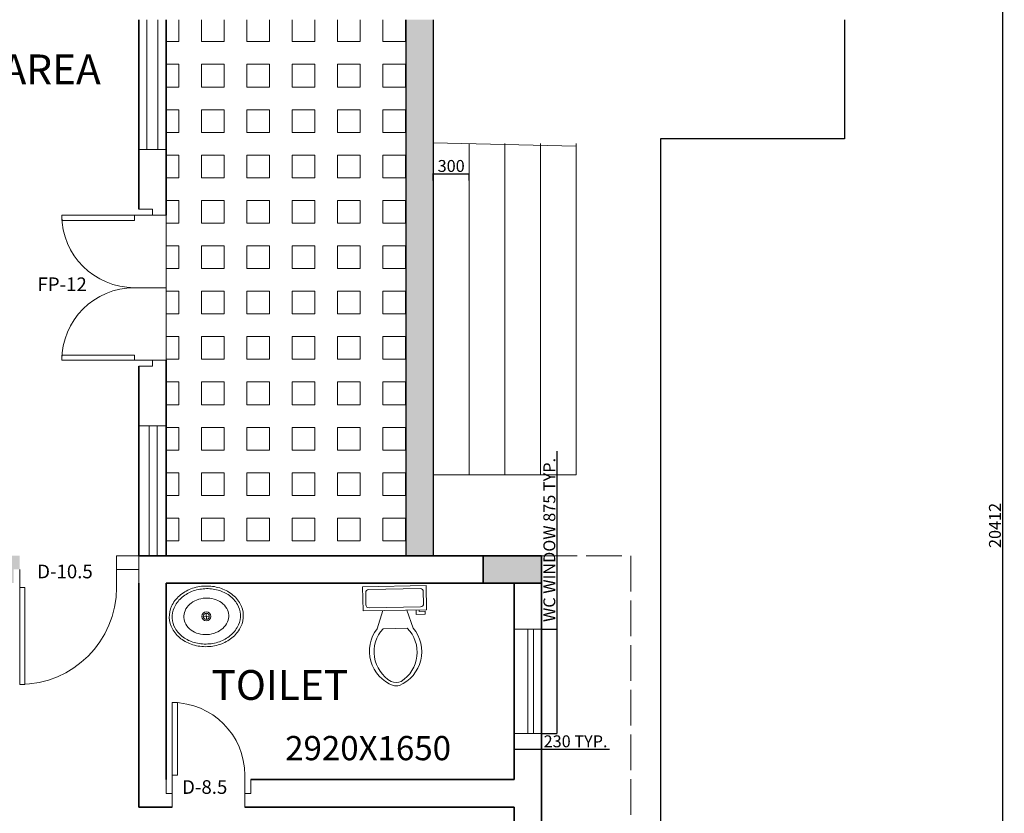
# Model space of a CAD drawing. Units: millimetres. Extents: x -17016 to 4866, y -18325 to 4338.
# Tile 4 of 5: x -3399 to 4866, y -9462 to -2799. Entities that reach past the tile are written whole.
import ezdxf

# ---------------------------------------------------------------- set-up
doc = ezdxf.new("R2010")
doc.units = ezdxf.units.MM
doc.header["$LTSCALE"] = 5
doc.linetypes.add('ACAD_ISO02W100', pattern=[15, 12, -3])
for name, color, linetype, lineweight in [('A-ANNO-DIMS', 2, 'Continuous', 18), ('A-ANNO-IDEN', 3, 'Continuous', 18), ('A-AREA-IDEN', 7, 'Continuous', 25), ('A-COLS', 7, 'Continuous', 35), ('A-COLS-PATT', 252, 'Continuous', 13), ('A-DOOR', 3, 'Continuous', 18), ('A-FLOR-FIXT', 9, 'Continuous', 18), ('A-FLOR-OTLN', 8, 'Continuous', 25), ('A-FLOR-PATT', 252, 'Continuous', 13), ('A-FLOR-STRS', 7, 'Continuous', 18), ('A-GLAZ', 4, 'Continuous', 18), ('A-ROOF-OVHD', 8, 'ACAD_ISO02W100', 13), ('A-WALL', 7, 'Continuous', 35)]:
    doc.layers.add(name, color=color, linetype=linetype, lineweight=lineweight)
doc.styles.get("Standard").update_dxf_attribs({"font": 'arial.ttf'})
doc.dimstyles.new('Copy of ISO-25', dxfattribs={"dimtxt": 100, "dimasz": 2.5, "dimexe": 1.25, "dimexo": 0.625, "dimtad": 1, "dimdec": 0, "dimtxsty": 'Standard', "dimcen": 2.5, "dimadec": 0, "dimazin": 0, "dimtfac": 1, "dimtdec": 0, "dimtmove": 0, "dimatfit": 3, "dimfxl": 1, "dimarcsym": 0})

# ---------------------------------------------------------------- blocks, each defined once
blk = doc.blocks.new('*U3')
for p, q in [((0, 0), (0, -6)), ((24, 0), (24, -6))]:
    blk.add_line(p, q)
blk.add_lwpolyline([(0, 0), (0, 24), (1.75, 24), (1.75, 0)], close=True)
blk.add_arc((0, 0), 24, 0, 90)
blk = doc.blocks.new('Sink - Oval top')
for p, q in [((-1, 0), (1, 0)), ((0, 1), (0, -1))]:
    blk.add_line(p, q)
for points in [[(-12.23, 0.39, 0.117634), (-11.46, -3.36, 0.104469), (-8.88, -6.8, 0.090016), (-5.08, -9.07, 0.08192), (-0.32, -10.02, 0.08192), (4.49, -9.38, 0.090016), (8.42, -7.36, 0.104469), (11.22, -4.09, 0.117634), (12.23, -0.39, 0.117634), (11.46, 3.36, 0.104469), (8.88, 6.8, 0.090016), (5.08, 9.07, 0.08192), (0.32, 10.02, 0.08192), (-4.49, 9.38, 0.090016), (-8.42, 7.36, 0.104469), (-11.22, 4.09, 0.117634)], [(-11.29, 0.16, 0.118622), (-10.52, -3.25, 0.104678), (-8.07, -6.36, 0.089562), (-4.54, -8.37, 0.081185), (-0.13, -9.15, 0.081185), (4.3, -8.49, 0.089562), (7.89, -6.58, 0.104678), (10.42, -3.55, 0.118622), (11.29, -0.16, 0.118622), (10.52, 3.25, 0.104678), (8.07, 6.36, 0.089562), (4.54, 8.37, 0.081185), (0.13, 9.15, 0.081185), (-4.3, 8.49, 0.089562), (-7.89, 6.58, 0.104678), (-10.42, 3.55, 0.118622)], [(-7.42, 0.08, 0.118283), (-6.91, -2.17, 0.104607), (-5.29, -4.21, 0.089718), (-2.97, -5.53, 0.081436), (-0.07, -6.04, 0.081436), (2.84, -5.59, 0.089718), (5.2, -4.33, 0.104607), (6.86, -2.32, 0.118283), (7.42, -0.08, 0.118283), (6.91, 2.17, 0.104607), (5.29, 4.21, 0.089718), (2.97, 5.53, 0.081436), (0.07, 6.04, 0.081436), (-2.84, 5.59, 0.089718), (-5.2, 4.33, 0.104607), (-6.86, 2.32, 0.118283)]]:
    blk.add_lwpolyline(points, format="xyb", close=True)
for radius in [1.5, 1]:
    blk.add_circle((0, 0), radius)
blk = doc.blocks.new('*U13')
for p, q in [((9.5, -6), (9.5, -2)), ((-10, -8.5), (-8, -8.5)), ((-10, -9.5), (-10, -8.5)), ((-7, -9.5), (-10, -9.5)), ((-8, -8.5), (-8, -8)), ((-7, -8), (-7, -9.5)), ((-4, -8), (-6, -14)), ((4, -8), (6, -14)), ((4, -14), (-4, -14))]:
    blk.add_line(p, q)
blk.add_lwpolyline([(10.5, -8), (10.5, 0), (-10.5, 0), (-10.5, -8)], close=True)
for points in [[(-9.5, -2), (-9.5, -6)], [(8.5, -1), (-8.5, -1)], [(-8.5, -7), (8.5, -7)]]:
    blk.add_lwpolyline(points)
for centre, radius, start, end in [((-8.62, -1.88), 0.884, 81.8699, 188.1301), ((8.62, -1.88), 0.884, 351.8699, 98.1301), ((-8.62, -6.12), 0.884, 171.8699, 278.1301), ((8.62, -6.12), 0.884, 261.8699, 8.1301), ((3.52, -21.58), 12.17, 141.4691, 247.9714), ((4.2, -21.82), 11.33, 136.3677, 238.9468), ((-3.52, -21.58), 12.17, 292.0284, 38.5307), ((-4.2, -21.82), 11.33, 301.053, 43.6321), ((0, -27.88), 4, 245.7318, 294.2682), ((0, -29), 4, 254.8605, 285.1395)]:
    blk.add_arc(centre, radius, start, end)
blk = doc.blocks.new('*U2')
for p, q in [((0, 0), (0, -6)), ((32, 0), (32, -6))]:
    blk.add_line(p, q)
blk.add_lwpolyline([(0, 0), (0, 32), (1.75, 32), (1.75, 0)], close=True)
blk.add_arc((0, 0), 32, 0, 90)
blk = doc.blocks.new('*D16')
at = {"layer": 'A-ANNO-DIMS', "color": 0, "lineweight": -2, "ltscale": 5, "transparency": 16777216}
for p, q in [((72.8, -4147.8), (72.8, -4090.5)), ((75.3, -4091.8), (370.2, -4091.8)), ((372.7, -4147.8), (372.7, -4090.5))]:
    blk.add_line(p, q, dxfattribs=at)
at = {"layer": 'A-ANNO-DIMS', "color": 0, "ltscale": 5, "transparency": 16777216}
for points in [[(75.3, -4091.4), (75.3, -4092.2), (72.8, -4091.8)], [(370.2, -4091.4), (370.2, -4092.2), (372.7, -4091.8)]]:
    blk.add_solid(points, dxfattribs=at)
at = {"layer": 'Defpoints', "color": 0, "ltscale": 5, "transparency": 16777216}
for p in [(372.7, -4091.8), (72.8, -4148.4), (372.7, -4148.4)]:
    blk.add_point(p, dxfattribs=at)
at = {"layer": 'A-ANNO-DIMS', "color": 0, "ltscale": 5, "transparency": 16777216, "insert": (222.8, -4040.1), "char_height": 100, "attachment_point": 5}
blk.add_mtext('300', dxfattribs=at)
blk = doc.blocks.new('WIN-TOILET-875')
for p, q in [((0, 874.8), (230, 874.8)), ((115, 874.8), (115, 0)), ((164.3, 874.8), (164.3, 0)), ((0, 0), (230, 0))]:
    blk.add_line(p, q)
blk = doc.blocks.new('*D34')
at = {"layer": 'A-ANNO-DIMS', "color": 0, "lineweight": -2, "ltscale": 5, "transparency": 16777216}
for p, q in [((1112, -7915.9), (1112, -6420.3)), ((981.4, -7915.9), (1113.3, -7915.9)), ((1112, -8788.2), (1112, -7918.4)), ((981.4, -8790.7), (1113.3, -8790.7))]:
    blk.add_line(p, q, dxfattribs=at)
at = {"layer": 'A-ANNO-DIMS', "color": 0, "ltscale": 5, "transparency": 16777216}
for points in [[(1111.6, -7918.4), (1112.5, -7918.4), (1112, -7915.9)], [(1111.6, -8788.2), (1112.5, -8788.2), (1112, -8790.7)]]:
    blk.add_solid(points, dxfattribs=at)
at = {"layer": 'Defpoints', "color": 0, "ltscale": 5, "transparency": 16777216}
for p in [(980.8, -7915.9), (1112, -7915.9), (980.8, -8790.7)]:
    blk.add_point(p, dxfattribs=at)
at = {"layer": 'A-ANNO-DIMS', "color": 0, "ltscale": 5, "transparency": 16777216, "insert": (1059.7, -7166.8), "char_height": 100, "attachment_point": 5, "rotation": 90}
blk.add_mtext('WC WINDOW 875 TYP.', dxfattribs=at)
blk = doc.blocks.new('*D35')
at = {"layer": 'A-ANNO-DIMS', "color": 0, "lineweight": -2, "ltscale": 5, "transparency": 16777216}
for p, q in [((750.8, -8791.3), (750.8, -8923.1)), ((980.8, -8791.3), (980.8, -8923.1)), ((753.3, -8921.9), (978.3, -8921.9)), ((980.8, -8921.9), (1550.7, -8921.9))]:
    blk.add_line(p, q, dxfattribs=at)
at = {"layer": 'A-ANNO-DIMS', "color": 0, "ltscale": 5, "transparency": 16777216}
for points in [[(753.3, -8921.5), (753.3, -8922.3), (750.8, -8921.9)], [(978.3, -8921.5), (978.3, -8922.3), (980.8, -8921.9)]]:
    blk.add_solid(points, dxfattribs=at)
at = {"layer": 'Defpoints', "color": 0, "ltscale": 5, "transparency": 16777216}
for p in [(750.8, -8790.7), (980.8, -8790.7), (980.8, -8921.9)]:
    blk.add_point(p, dxfattribs=at)
at = {"layer": 'A-ANNO-DIMS', "color": 0, "ltscale": 5, "transparency": 16777216, "insert": (1267, -8870.2), "char_height": 100, "attachment_point": 5}
blk.add_mtext('230 TYP.', dxfattribs=at)
blk = doc.blocks.new('*D47')
at = {"layer": 'A-ANNO-DIMS', "color": 0, "lineweight": -2, "ltscale": 5, "transparency": 16777216}
for p, q in [((3524.2, 3160.9), (4853.2, 3160.9)), ((4851.9, 3158.4), (4851.9, -17248.3)), ((-3159.9, -17250.8), (4853.2, -17250.8))]:
    blk.add_line(p, q, dxfattribs=at)
at = {"layer": 'A-ANNO-DIMS', "color": 0, "ltscale": 5, "transparency": 16777216}
for points in [[(4851.5, 3158.4), (4852.3, 3158.4), (4851.9, 3160.9)], [(4851.5, -17248.3), (4852.3, -17248.3), (4851.9, -17250.8)]]:
    blk.add_solid(points, dxfattribs=at)
at = {"layer": 'Defpoints', "color": 0, "ltscale": 5, "transparency": 16777216}
for p in [(3523.6, 3160.9), (-3160.5, -17250.8), (4851.9, -17250.8)]:
    blk.add_point(p, dxfattribs=at)
at = {"layer": 'A-ANNO-DIMS', "color": 0, "ltscale": 5, "transparency": 16777216, "insert": (4800.2, -7045), "char_height": 100, "attachment_point": 5, "rotation": 90}
blk.add_mtext('20412', dxfattribs=at)

msp = doc.modelspace()

# ---------------------------------------------------------------- hatches: boundary and pattern name
at = {"layer": 'A-COLS-PATT', "ltscale": 5}
h = msp.add_hatch(color=256, dxfattribs=at)
h.dxf.hatch_style = 1
h.paths.add_polyline_path([(980.82, -7299.11), (490.82, -7299.11), (490.82, -7529.11), (980.82, -7529.11)])
h.paths.add_polyline_path([(-3449.18, -7414.11), (-3399.18, -7414.11), (-3399.18, -7299.11), (-3939.18, -7299.11), (-3939.18, -7529.11), (-3449.18, -7529.11)])
h.paths.add_polyline_path([(-8219.18, -7299.11), (-8709.18, -7299.11), (-8709.18, -7529.11), (-8219.18, -7529.11)])
h.paths.add_polyline_path([(-12649.22, -7299.11), (-13139.18, -7299.11), (-13139.18, -7529.11), (-12649.22, -7529.11)])
at = {"layer": 'A-FLOR-PATT'}
h = msp.add_hatch(dxfattribs=at)
h.set_pattern_fill('ANGLE', color=256, scale=25)
h.set_pattern_definition([(0, (-20162.07, -7174.37), (0, 174.625), [127, -47.625]), (90, (-20162.07, -7174.37), (-174.625, 1e-14), [127, -47.625])])
h.paths.add_polyline_path([(72.82, -2799.11), (-157.18, -2799.11), (-157.18, -7299.11), (72.82, -7299.11)])
h.paths.add_polyline_path([(-12231.38, -2799.11), (-12461.38, -2799.11), (-12461.38, -7299.11), (-12231.38, -7299.11)])
h = msp.add_hatch(dxfattribs=at)
h.set_pattern_fill('SQUARE', color=256, scale=60)
h.set_pattern_definition([(0, (-20162.07, -7174.37), (0, 190.5), [190.5, -190.5]), (90, (-20162.07, -7174.37), (-190.5, 1e-14), [190.5, -190.5])])
h.paths.add_polyline_path([(-157.18, -2799.11), (-436.38, -2799.11), (-2169.18, -2799.11), (-2169.18, -4439.51), (-2169.18, -5658.71), (-2169.18, -7299.11), (-157.18, -7299.11)])
h.paths.add_polyline_path([(-9989.18, -4439.51), (-9989.18, -2799.11), (-12231.38, -2799.11), (-12231.38, -7299.11), (-9989.18, -7299.11), (-9989.18, -5658.71)])

# ---------------------------------------------------------------- linework, layer by layer
at = {"layer": 'A-COLS', "ltscale": 5}
msp.add_line((490.82, -7534.51), (490.82, -7299.11), dxfattribs=at)
at = {"layer": 'A-DOOR'}
for p, q in [((-2284.18, -4389.51), (-2399.18, -4389.51)), ((-2284.18, -4439.51), (-2284.18, -4389.51)), ((-2284.18, -4439.51), (-2169.18, -4439.51)), ((-2169.18, -4439.51), (-2169.18, -5658.71)), ((-2399.18, -5049.11), (-2169.18, -5049.11)), ((-2284.18, -5658.71), (-2284.18, -5708.71)), ((-2284.18, -5658.71), (-2169.18, -5658.71)), ((-2284.18, -5708.71), (-2399.18, -5708.71)), ((-2586.38, -7414.11), (-2586.38, -7299.11)), ((-2399.18, -7299.11), (-2586.38, -7299.11)), ((-2399.18, -7299.11), (-2399.18, -7529.11)), ((-2586.38, -7414.11), (-2399.18, -7414.11)), ((-2169.18, -9179.11), (-2169.18, -9294.11)), ((-1459.58, -9294.11), (-1459.58, -9179.11)), ((-2169.18, -9294.11), (-2119.18, -9294.11)), ((-2119.18, -9294.11), (-2119.18, -9409.11)), ((-1509.58, -9294.11), (-1459.58, -9294.11)), ((-1509.58, -9294.11), (-1509.58, -9409.11))]:
    msp.add_line(p, q, dxfattribs=at)
at = {"layer": 'A-FLOR-OTLN'}
for p, q in [((-157.18, -2799.11), (-157.18, -7299.11)), ((72.82, -2799.11), (72.82, -7299.11))]:
    msp.add_line(p, q, dxfattribs=at)
at = {"layer": 'A-FLOR-OTLN', "ltscale": 5}
for p, q in [((3523.62, -2799.11), (3523.62, -3799.11)), ((3523.62, -3799.11), (1980.82, -3799.11)), ((1980.82, -3799.11), (1980.82, -13909.11))]:
    msp.add_line(p, q, dxfattribs=at)
at = {"layer": 'A-FLOR-STRS', "ltscale": 5}
for p, q in [((72.82, -3831.79), (1272.74, -3860.38)), ((372.74, -3838.93), (372.74, -6618.73)), ((672.74, -3838.93), (672.74, -6618.73)), ((972.74, -3838.93), (972.74, -6618.73)), ((1272.74, -3838.93), (1272.74, -6618.73)), ((1272.74, -6618.73), (72.82, -6618.73))]:
    msp.add_line(p, q, dxfattribs=at)
at = {"layer": 'A-GLAZ'}
for p, q in [((-2331.16, -2799.11), (-2331.16, -3889.51)), ((-2239.42, -2799.11), (-2239.42, -3889.51)), ((-2399.18, -3889.51), (-2169.18, -3889.51)), ((-2399.18, -6208.71), (-2169.18, -6208.71)), ((-2313.41, -6208.71), (-2313.41, -7299.11)), ((-2246.29, -6208.71), (-2246.29, -7299.11))]:
    msp.add_line(p, q, dxfattribs=at)
at = {"layer": 'A-ROOF-OVHD', "ltscale": 5}
for p, q in [((980.82, -7299.11), (1730.82, -7299.11)), ((1730.82, -7299.11), (1730.82, -13659.11))]:
    msp.add_line(p, q, dxfattribs=at)
at = {"layer": 'A-WALL'}
for p, q in [((-2399.18, -2799.11), (-2399.18, -4389.51)), ((-2169.18, -2799.11), (-2169.18, -4439.51)), ((-2169.18, -5658.71), (-2169.18, -7299.11)), ((-2399.18, -5708.71), (-2399.18, -7299.11)), ((980.82, -7299.11), (-2399.18, -7299.11)), ((980.82, -7299.11), (980.82, -12909.11)), ((-2399.18, -7529.11), (-2399.18, -9409.11)), ((980.82, -7529.11), (-2169.18, -7529.11)), ((-2169.18, -7529.11), (-2169.18, -9179.11)), ((750.82, -7529.11), (750.82, -9179.11)), ((750.82, -9179.11), (-1459.58, -9179.11)), ((-2119.18, -9409.11), (-2399.18, -9409.11)), ((750.82, -9409.11), (-1509.58, -9409.11)), ((750.82, -9409.11), (750.82, -12909.11))]:
    msp.add_line(p, q, dxfattribs=at)

# ---------------------------------------------------------------- block references
at = {"layer": 'A-DOOR', "yscale": 25.4, "zscale": 25.4}
for name, p, xscale, rotation in [('*U3', (-2436.58, -4439.51), -25.4, 90), ('*U3', (-2436.58, -5658.71), 25.4, 90.00000000000003), ('*U2', (-3399.18, -7566.51), -25.4, 180)]:
    msp.add_blockref(name, p, dxfattribs=dict(at, xscale=xscale, rotation=rotation))
at = {"layer": 'A-DOOR', "xscale": 25.4, "yscale": 25.4, "zscale": 25.4}
msp.add_blockref('*U3', (-2119.18, -9141.71), dxfattribs=at)
at = {"layer": 'A-FLOR-FIXT', "yscale": 25.4, "zscale": 25.4}
for name, p, xscale, rotation in [('Sink - Oval top', (-1832.98, -7808.1), 25.4, 3.833934461057109), ('*U13', (-253.94, -7554.18), -25.4, 1.060997950081761)]:
    msp.add_blockref(name, p, dxfattribs=dict(at, xscale=xscale, rotation=rotation))
at = {"layer": 'A-GLAZ'}
msp.add_blockref('WIN-TOILET-875', (750.82, -8790.67), dxfattribs=at)

# ---------------------------------------------------------------- texts
at = {"layer": 'A-ANNO-IDEN', "ltscale": 5}
for s, p in [('FP-12', (-3249.8, -5077.65)), ('D-10.5', (-3252.41, -7488.78)), ('D-8.5', (-2035.88, -9298.36))]:
    msp.add_text(s, height=114.837, dxfattribs=at).set_placement(p)
at = {"layer": 'A-AREA-IDEN', "ltscale": 5}
for s, height, p in [('LIVING/DINING AREA', 250, (-5986.71, -3341.18)), ('TOILET', 250, (-1789.21, -8509.31)), ('2920X1650', 203.546, (-1170.53, -9015.99))]:
    msp.add_text(s, height=height, dxfattribs=at).set_placement(p)

# ---------------------------------------------------------------- dimensions: what is measured, and where the dimension line sits
at = {"layer": 'A-ANNO-DIMS', "ltscale": 5}
dim = msp.add_linear_dim(base=(4851.91, -17250.83), p1=(3523.62, 3160.89), p2=(-3160.48, -17250.83), angle=90, dimstyle='Copy of ISO-25', override={"dimdec": 0, "dimlfac": 1, "dimrnd": 0, "dimzin": 0, "dimdsep": 46, "dimlunit": 2}, dxfattribs=at)
dim.commit()
dim.dimension.update_dxf_attribs({"geometry": '*D47', "text_midpoint": (4800.22, -7044.97)})
dim = msp.add_linear_dim(base=(372.74, -4091.77), p1=(72.82, -4148.4), p2=(372.74, -4148.4), dimstyle='Copy of ISO-25', override={"dimclrd": 0, "dimclre": 0, "dimclrt": 0}, dxfattribs=at)
dim.commit()
dim.dimension.update_dxf_attribs({"geometry": '*D16', "text_midpoint": (222.78, -4040.06)})
dim = msp.add_linear_dim(base=(1112.04, -7915.9), p1=(980.82, -8790.67), p2=(980.82, -7915.9), angle=90, text='WC WINDOW <> TYP.', dimstyle='Copy of ISO-25', override={"dimdec": 0, "dimlfac": 1, "dimrnd": 0, "dimzin": 0, "dimdsep": 46, "dimlunit": 2}, dxfattribs=at)
dim.commit()
dim.dimension.update_dxf_attribs({"geometry": '*D34', "text_midpoint": (1059.67, -7166.84)})
dim = msp.add_linear_dim(base=(980.82, -8921.89), p1=(750.82, -8790.67), p2=(980.82, -8790.67), text='<> TYP.', dimstyle='Copy of ISO-25', override={"dimdec": 0, "dimlfac": 1, "dimrnd": 0, "dimzin": 0, "dimdsep": 46, "dimlunit": 2}, dxfattribs=at)
dim.commit()
dim.dimension.update_dxf_attribs({"geometry": '*D35', "text_midpoint": (1267.03, -8870.17)})

doc.saveas('drawing.dxf')
